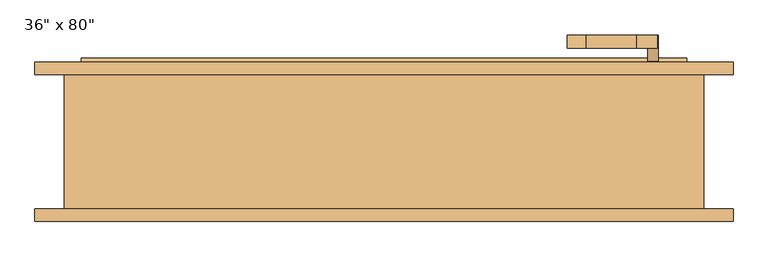
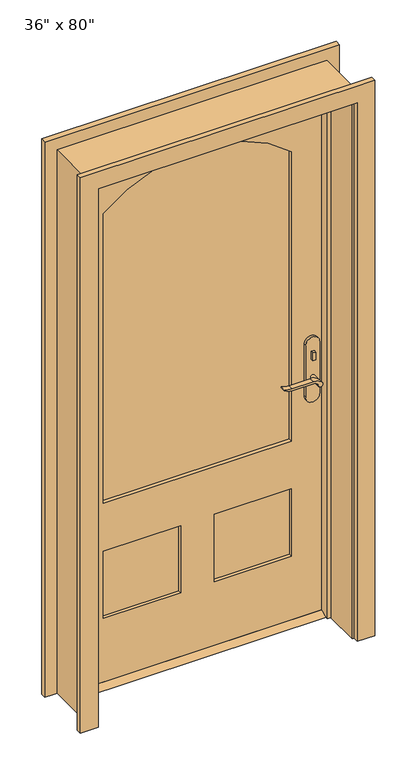
"""IFC4 building model written with IfcOpenShell, lengths in millimetres: door geometry."""

from ifc_helpers import new_model, si_unit, point, frame, frame_2d, origin, place, context, project, spatial, polyline, circle_curve, trimmed, segment, composite_curve, outline, extrude, faceted_brep, source, transform, mapped, element, save


def door_1768e003(model_context):
    return source(origin(), model_context, "Body", "SolidModel", [
        extrude(outline(polyline([(63.5, 12.7), (98.425, 12.7), (123.825, 0.0), (38.1, 0.0), (63.5, 12.7)])), frame((-457.2, 0.0, 0.0), z_axis=(1.0, 0.0, 0.0), x_axis=(0.0, 1.0, 0.0)), (0.0, 0.0, 1.0), 914.4),
        extrude(outline(polyline([(411.4, 43.5), (401.4, 43.5), (401.4, 53.5), (411.4, 53.5), (411.4, 43.5)])), frame((0.0, 0.0, 981.9), z_axis=(0.0, 0.0, 1.0), x_axis=(1.0, 0.0, 0.0)), (0.0, 0.0, 1.0), 30.0),
        extrude(outline(composite_curve([segment(trimmed(circle_curve(frame_2d((996.9, 406.4)), 8.0), [point((996.9, 398.4))], [point((996.9, 414.4))], False, "CARTESIAN"), True, "CONTINUOUS"), segment(trimmed(circle_curve(frame_2d((996.9, 406.4)), 8.0), [point((996.9, 414.4))], [point((996.9, 398.4))], False, "CARTESIAN"), True, "CONTINUOUS")], self_intersect=False)), frame((0.0, 108.425, 0.0), z_axis=(0.0, 1.0, 0.0), x_axis=(0.0, 0.0, 1.0)), (0.0, 0.0, 1.0), 10.0),
        extrude(outline(composite_curve([segment(trimmed(circle_curve(frame_2d((897.1555521, 382.7324871)), 37.2832219), [point((919.0523287, 412.9081363))], [point((934.4, 381.0325667))], False, "CARTESIAN"), True, "CONTINUOUS"), segment(polyline([(934.4, 381.0325667), (934.4, 304.7564091)]), True, "CONTINUOUS"), segment(trimmed(circle_curve(frame_2d((1017.6850638, 304.8227909)), 83.2850902), [point((934.4, 304.7564091))], [point((939.4, 276.4))], True, "CARTESIAN"), True, "CONTINUOUS"), segment(polyline([(939.4, 276.4), (936.6135558, 276.4)]), True, "CONTINUOUS"), segment(trimmed(circle_curve(frame_2d((986.6709207, 308.3396612)), 59.3791355), [point((936.6135558, 276.4))], [point((927.4, 304.7564091))], False, "CARTESIAN"), True, "CONTINUOUS"), segment(polyline([(927.4, 304.7564091), (927.4, 381.0138099)]), True, "CONTINUOUS"), segment(trimmed(circle_curve(frame_2d((909.2738613, 381.0138099)), 18.1261387), [point((927.4, 381.0138099))], [point((914.4, 398.4))], True, "CARTESIAN"), True, "CONTINUOUS"), segment(trimmed(circle_curve(frame_2d((914.4, 406.4)), 8.0), [point((914.4, 398.4))], [point((919.0523287, 412.9081363))], False, "CARTESIAN"), True, "CONTINUOUS")], self_intersect=False)), frame((0.0, 3.5, 0.0), z_axis=(0.0, 1.0, 0.0), x_axis=(0.0, 0.0, 1.0)), (0.0, 0.0, 1.0), 20.0),
        extrude(outline(composite_curve([segment(trimmed(circle_curve(frame_2d((914.4, 406.4)), 8.0), [point((914.3999903, 398.4))], [point((919.0523287, 412.9081363))], False, "CARTESIAN"), True, "CONTINUOUS"), segment(trimmed(circle_curve(frame_2d((897.1555521, 382.7324871)), 37.2832219), [point((919.0523287, 412.9081363))], [point((934.4, 381.0325667))], False, "CARTESIAN"), True, "CONTINUOUS"), segment(polyline([(934.4, 381.0325667), (934.4, 304.7564091)]), True, "CONTINUOUS"), segment(trimmed(circle_curve(frame_2d((1017.6850638, 304.8227909)), 83.2850902), [point((934.4, 304.7564091))], [point((939.4, 276.4))], True, "CARTESIAN"), True, "CONTINUOUS"), segment(polyline([(939.4, 276.4), (936.6135558, 276.4)]), True, "CONTINUOUS"), segment(trimmed(circle_curve(frame_2d((986.6709207, 308.3396612)), 59.3791355), [point((936.6135558, 276.4))], [point((927.4, 304.7564091))], False, "CARTESIAN"), True, "CONTINUOUS"), segment(polyline([(927.4, 304.7564091), (927.4, 381.0138122)]), True, "CONTINUOUS"), segment(trimmed(circle_curve(frame_2d((909.2738682, 381.0138122)), 18.1261318), [point((927.4, 381.0138122))], [point((914.3999903, 398.4))], True, "CARTESIAN"), True, "CONTINUOUS")], self_intersect=False)), frame((0.0, 138.425, 0.0), z_axis=(0.0, 1.0, 0.0), x_axis=(0.0, 0.0, 1.0)), (0.0, 0.0, 1.0), 20.0),
        extrude(outline(composite_curve([segment(trimmed(circle_curve(frame_2d((914.4, 406.4)), 8.0), [point((914.4, 398.4))], [point((914.4, 414.4))], False, "CARTESIAN"), True, "CONTINUOUS"), segment(trimmed(circle_curve(frame_2d((914.4, 406.4)), 8.0), [point((914.4, 414.4))], [point((914.4, 398.4))], False, "CARTESIAN"), True, "CONTINUOUS")], self_intersect=False)), frame((0.0, 23.5, 0.0), z_axis=(0.0, 1.0, 0.0), x_axis=(0.0, 0.0, 1.0)), (0.0, 0.0, 1.0), 30.0),
        extrude(outline(composite_curve([segment(trimmed(circle_curve(frame_2d((914.4, 406.4)), 8.0), [point((914.4, 398.4))], [point((914.4, 414.4))], False, "CARTESIAN"), True, "CONTINUOUS"), segment(trimmed(circle_curve(frame_2d((914.4, 406.4)), 8.0), [point((914.4, 414.4))], [point((914.4, 398.4))], False, "CARTESIAN"), True, "CONTINUOUS")], self_intersect=False)), frame((0.0, 108.425, 0.0), z_axis=(0.0, 1.0, 0.0), x_axis=(0.0, 0.0, 1.0)), (0.0, 0.0, 1.0), 30.0),
        extrude(outline(composite_curve([segment(polyline([(844.4, 431.4), (1039.4, 431.4)]), True, "CONTINUOUS"), segment(trimmed(circle_curve(frame_2d((1039.4, 406.4)), 25.0), [point((1039.4, 431.4))], [point((1039.4, 381.4))], False, "CARTESIAN"), True, "CONTINUOUS"), segment(polyline([(1039.4, 381.4), (844.4, 381.4)]), True, "CONTINUOUS"), segment(trimmed(circle_curve(frame_2d((844.4, 406.4)), 25.0), [point((844.4, 381.4))], [point((844.4, 431.4))], False, "CARTESIAN"), True, "CONTINUOUS")], self_intersect=False)), frame((0.0, 53.5, 0.0), z_axis=(0.0, 1.0, 0.0), x_axis=(0.0, 0.0, 1.0)), (0.0, 0.0, 1.0), 10.0),
        extrude(outline(composite_curve([segment(polyline([(844.4, 431.4), (1039.4, 431.4)]), True, "CONTINUOUS"), segment(trimmed(circle_curve(frame_2d((1039.4, 406.4)), 25.0), [point((1039.4, 431.4))], [point((1039.4, 381.4))], False, "CARTESIAN"), True, "CONTINUOUS"), segment(polyline([(1039.4, 381.4), (844.4, 381.4)]), True, "CONTINUOUS"), segment(trimmed(circle_curve(frame_2d((844.4, 406.4)), 25.0), [point((844.4, 381.4))], [point((844.4, 431.4))], False, "CARTESIAN"), True, "CONTINUOUS")], self_intersect=False)), frame((0.0, 98.425, 0.0), z_axis=(0.0, 1.0, 0.0), x_axis=(0.0, 0.0, 1.0)), (0.0, 0.0, 1.0), 10.0),
        extrude(outline(polyline([(2032.0, -457.2), (12.7, -457.2), (12.7, 457.2), (2032.0, 457.2), (2032.0, -457.2)]), holes=[composite_curve([segment(polyline([(688.975, -336.55), (1784.35, -336.55)]), True, "CONTINUOUS"), segment(trimmed(circle_curve(frame_2d((1401.92125, 0.0)), 509.42875), [point((1784.35, -336.55))], [point((1784.35, 336.55))], True, "CARTESIAN"), True, "CONTINUOUS"), segment(polyline([(1784.35, 336.55), (688.975, 336.55), (688.975, -336.55)]), True, "CONTINUOUS")], self_intersect=False), polyline([(508.0, -60.325), (254.0, -60.325), (254.0, -336.55), (508.0, -336.55), (508.0, -60.325)]), polyline([(508.0, 336.55), (254.0, 336.55), (254.0, 60.325), (508.0, 60.325), (508.0, 336.55)])]), frame((0.0, 63.5, 0.0), z_axis=(0.0, 1.0, 0.0), x_axis=(0.0, 0.0, 1.0)), (0.0, 0.0, 1.0), 34.925),
        faceted_brep([(482.6, 98.425, 0.0), (482.6, -104.775, 0.0), (457.2, -104.775, 0.0), (457.2, 28.575, 0.0), (444.5, 28.575, 0.0), (444.5, 63.5, 0.0), (457.2, 63.5, 0.0), (457.2, 98.425, 0.0), (482.6, 98.425, 2057.4), (482.6, -104.775, 2057.4), (-482.6, -104.775, 2057.4), (-482.6, -104.775, 0.0), (-457.2, -104.775, 0.0), (-457.2, -104.775, 2032.0), (457.2, -104.775, 2032.0), (457.2, 28.575, 2032.0), (-457.2, 28.575, 2032.0), (-457.2, 28.575, 0.0), (-444.5, 28.575, 0.0), (-444.5, 28.575, 2019.3), (444.5, 28.575, 2019.3), (444.5, 63.5, 2019.3), (-444.5, 63.5, 2019.3), (-444.5, 63.5, 0.0), (-457.2, 63.5, 0.0), (-457.2, 63.5, 2032.0), (457.2, 63.5, 2032.0), (457.2, 98.425, 2032.0), (-457.2, 98.425, 2032.0), (-457.2, 98.425, 0.0), (-482.6, 98.425, 0.0), (-482.6, 98.425, 2057.4)], [[[0, 1, 2, 3, 4, 5, 6, 7]], [[1, 0, 8, 9]], [[2, 1, 9, 10, 11, 12, 13, 14]], [[3, 2, 14, 15]], [[4, 3, 15, 16, 17, 18, 19, 20]], [[5, 4, 20, 21]], [[6, 5, 21, 22, 23, 24, 25, 26]], [[7, 6, 26, 27]], [[0, 7, 27, 28, 29, 30, 31, 8]], [[9, 8, 31, 10]], [[15, 14, 13, 16]], [[21, 20, 19, 22]], [[27, 26, 25, 28]], [[30, 29, 24, 23, 18, 17, 12, 11]], [[10, 31, 30, 11]], [[16, 13, 12, 17]], [[22, 19, 18, 23]], [[28, 25, 24, 29]]]),
        extrude(outline(polyline([(-60.325, 75.1416667), (-336.55, 75.1416667), (-336.55, 86.7833333), (-60.325, 86.7833333), (-60.325, 75.1416667)])), frame((0.0, 0.0, 254.0), z_axis=(0.0, 0.0, 1.0), x_axis=(1.0, 0.0, 0.0)), (0.0, 0.0, 1.0), 254.0),
        extrude(outline(polyline([(336.55, 75.1416667), (60.325, 75.1416667), (60.325, 86.7833333), (336.55, 86.7833333), (336.55, 75.1416667)])), frame((0.0, 0.0, 254.0), z_axis=(0.0, 0.0, 1.0), x_axis=(1.0, 0.0, 0.0)), (0.0, 0.0, 1.0), 254.0),
        extrude(outline(composite_curve([segment(polyline([(688.975, -336.55), (688.975, 336.55), (1784.35, 336.55)]), True, "CONTINUOUS"), segment(trimmed(circle_curve(frame_2d((1401.92125, 0.0)), 509.42875), [point((1784.35, 336.55))], [point((1784.35, -336.55))], False, "CARTESIAN"), True, "CONTINUOUS"), segment(polyline([(1784.35, -336.55), (688.975, -336.55)]), True, "CONTINUOUS")], self_intersect=False)), frame((0.0, 77.47, 0.0), z_axis=(0.0, 1.0, 0.0), x_axis=(0.0, 0.0, 1.0)), (0.0, 0.0, 1.0), 6.985),
        extrude(outline(polyline([(0.0, -527.05), (0.0, -463.55), (2038.35, -463.55), (2038.35, 463.55), (0.0, 463.55), (0.0, 527.05), (2101.85, 527.05), (2101.85, -527.05), (0.0, -527.05)])), frame((0.0, -123.825, 0.0), z_axis=(0.0, 1.0, 0.0), x_axis=(0.0, 0.0, 1.0)), (0.0, 0.0, 1.0), 19.05),
        extrude(outline(polyline([(0.0, -527.05), (0.0, -463.55), (2038.35, -463.55), (2038.35, 463.55), (0.0, 463.55), (0.0, 527.05), (2101.85, 527.05), (2101.85, -527.05), (0.0, -527.05)])), frame((0.0, 98.425, 0.0), z_axis=(0.0, 1.0, 0.0), x_axis=(0.0, 0.0, 1.0)), (0.0, 0.0, 1.0), 19.05),
    ])


if __name__ == "__main__":
    model = new_model("IFC4")
    model_context = context("Model", 3, world=origin())
    ifc_project = project(units=[si_unit("LENGTHUNIT", "METRE", prefix="MILLI")], contexts=[model_context])
    site = spatial("IfcSite", under=ifc_project)
    building = spatial("IfcBuilding", under=site)
    placement = place(None, origin())
    door_shape = door_1768e003(model_context)
    element("IfcDoor", 1, ObjectType="36\" x 80\"", at=placement, inside=building, context=model_context, shape_type="MappedRepresentation", body=[
        mapped(door_shape, transform((0.0, 0.0, 0.0), x_axis=(1.0, 0.0, 0.0), y_axis=(0.0, 1.0, 0.0), z_axis=(0.0, 0.0, 1.0))),
    ])
    save(model, "model.ifc")

# Revit data of these elements
# Type "36\" x 80\""
#   Type Mark = "15"
#   Assembly Code = "B2030100"
#   Analytic Construction = "French door, wood frame with single glass"
#   Threshold Offset [instance default] = 0' - 0 1/2"
#   Thickness = 0' - 1 3/8"
#   Thermal Resistance (R) = 1.0696 (h·ft²·°F)/BTU
#   Swing Angle [instance default] = 90.00°
#   Stiles = 0' - 4 3/4"
#   Rough Width = 3' - 2"
#   Rough Height = 6' - 9"
#   Radius = 1' - 8.05625"
#   Lock Rail = 0' - 7 1/8"
#   Height = 6' - 8"
#   Width = 3' - 0"
#   Heat Transfer Coefficient (U) = 0.9350 BTU/(h·ft²·°F)
#   Door Offset [instance default] = 0' - 0"
#   Bottom Rail = 0' - 9 1/2"
#   Threshold [instance default] = yes
#   Function = 1
#   Exterior Trim [instance default] = yes
#   Trim Material = Cherry
#   Threshold Material = Cherry
#   Panel Material = Cherry
#   Glazing = Glass
#   Frame Material = Cherry
#   Door Handle Material = Aluminum
#   Visual Light Transmittance = 0
#   Solar Heat Gain Coefficient = 0
#   Wall Closure = (empty or 0)
#   Construction Type = (empty or 0)
# Element 1 (IfcDoor, "36\" x 80\"")
#   Materials on its faces: "Cherry", "Aluminum", "Glass"
# Materials
#   "Cherry": class "Wood", colour RGB 226 177 128, transparency 0, Description = "Prunus Serotina", Cost = 0
#   "Glass": class "Glass", colour RGB 0 128 192, transparency 0.75, Description = "Soda Lime Glass", Cost = 0
#   "Aluminum": class "Metal", colour RGB 247 247 247, transparency 0, Description = "Aluminum 6061", Cost = 0
